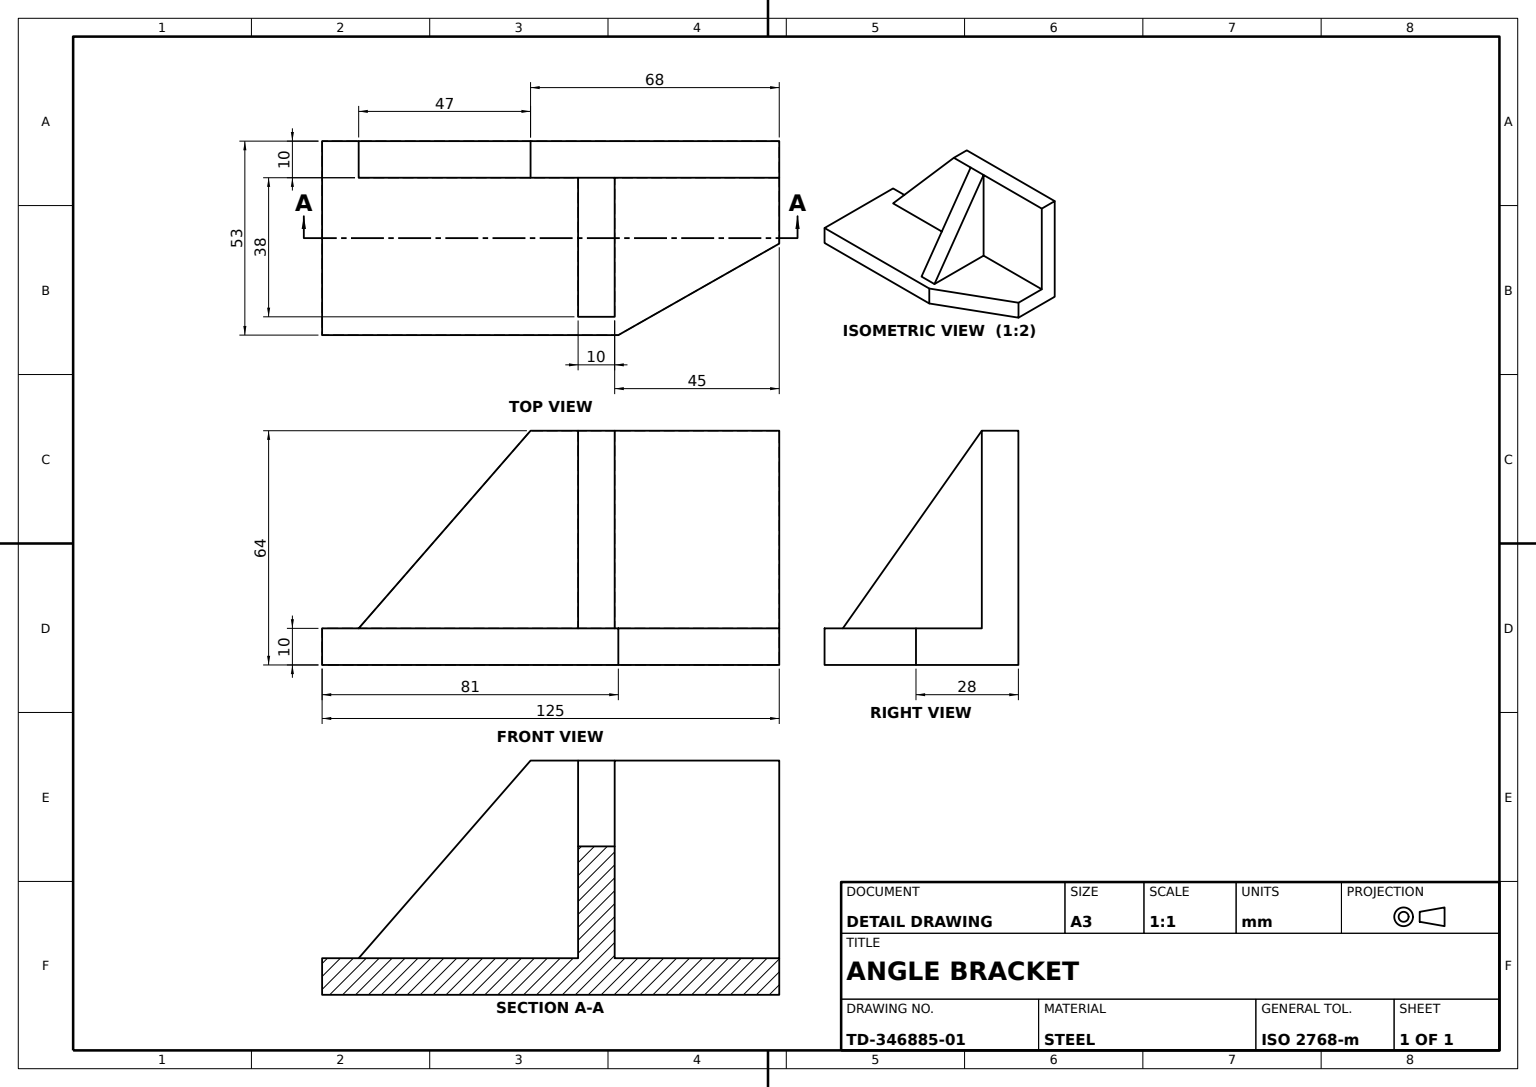
SolidWorks part; units mm, degrees
material "Plain Carbon Steel"
ref_plane "Front Plane" through (0, 0, 0) normal (0, 0, 1) x (1, 0, 0)
ref_plane "Top Plane" through (0, 0, 0) normal (0, 1, 0) x (1, 0, 0)
ref_plane "Right Plane" through (0, 0, 0) normal (1, 0, 0) x (0, 0, -1)
sketch "Base Plate Profile" plane through (0, 0, 0) normal (0, 1, 0) x (1, 0, 0)
  line L4 (0, 0) -> (81, 0)
  line L5 (81, 0) -> (125, 25)
  line L6 (125, 25) -> (125, 53)
  line L7 (125, 53) -> (0, 53)
  line L8 (0, 53) -> (0, 0)
  dimension "D1" = 81
  dimension "D2" = 125
  dimension "D3" = 53
  dimension "D4" = 28
extrude "Base Plate" add sketch "Base Plate Profile" along normal mid plane 10
sketch "Raised Pad Profile" plane through (0, 0, -53) normal (0, 0, -1) x (-1, 0, 0)
  line L0 (-125, 5) -> (-10, 5)
  line L1 (-125, 5) -> (0, 5) construction
  line L3 (-125, 5) -> (-125, 59)
  line L4 (-125, 59) -> (-57, 59)
  line L5 (-57, 59) -> (-10, 5)
  dimension "D1" = 54
  dimension "D2" = 68
  dimension "D3" = 47
extrude "Raised Pad" add sketch "Raised Pad Profile" against normal blind 10 contours L5 L0 L3 L4
sketch "Upright Wall Profile" plane through (0, 5, 0) normal (0, 1, 0) x (1, 0, 0)
  line L1 (125, 43) -> (10, 43) construction
  line L2 (80, 43) -> (80, 5)
  line L3 (80, 5) -> (70, 5)
  line L4 (70, 5) -> (70, 43)
  line L5 (70, 43) -> (80, 43)
  dimension "D1" = 70.1783
  dimension "D2" = 10
  dimension "D3" = 38
extrude "Upright Wall" add sketch "Upright Wall Profile" along normal blind 54
sketch "Gusset Cut Profile" plane through (80, 0, 0) normal (1, 0, 0) x (0, 0, -1)
  line L0 (43, 59) -> (5, 5)
  line L1 (5, 5) -> (43, 5) construction
  line L2 (0, 5) -> (25, 5) construction
  line L3 (5, 5) -> (5, 59)
  line L4 (5, 59) -> (43, 59)
extrude "Gusset Cut" cut sketch "Gusset Cut Profile" against normal blind 10
